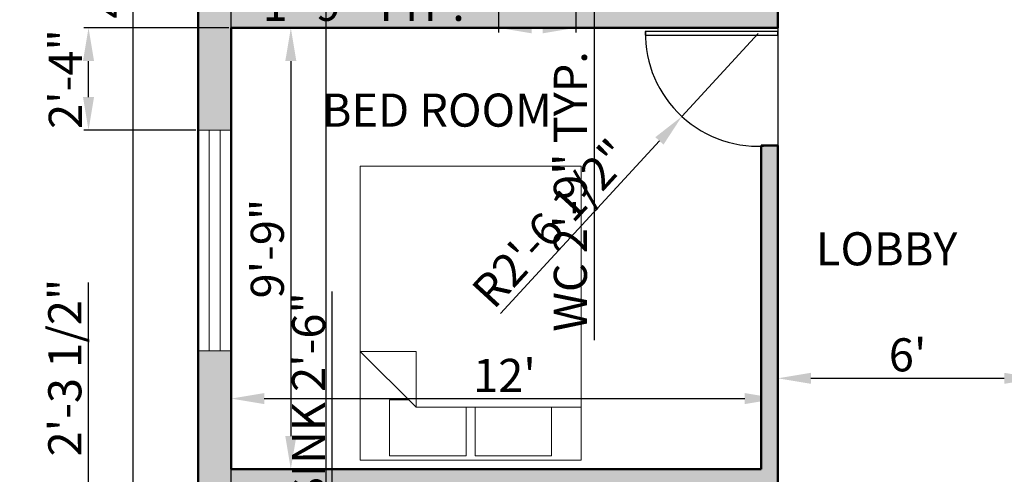
# Model space of a CAD drawing. Units: inches. Extents: x 875413 to 876020, y 447446 to 448210.
# Tile 2 of 8: x 875413 to 875681, y 447671 to 447795. Entities that reach past the tile are written whole.
import ezdxf

# ---------------------------------------------------------------- set-up
doc = ezdxf.new("R2010")
doc.units = ezdxf.units.IN
for name, color, linetype, lineweight in [('A-ANNO-DIMS', 2, 'Continuous', 13), ('A-AREA-IDEN', 7, 'Continuous', 25), ('A-DOOR', 3, 'Continuous', 25), ('A-FURN', 8, 'Continuous', 18), ('A-GLAZ', 4, 'Continuous', 20), ('A-WALL', 7, 'Continuous', 50)]:
    doc.layers.add(name, color=color, linetype=linetype, lineweight=lineweight)
doc.layers.add('A-WALL-PATT', color=18, linetype='Continuous', lineweight=13, true_color=0x000000)
doc.styles.get("Standard").update_dxf_attribs({"font": 'arial.ttf'})
doc.dimstyles.new('ISO-25', dxfattribs={"dimtxt": 9, "dimasz": 9, "dimexe": 1.25, "dimexo": 0.625, "dimtad": 1, "dimdec": 1, "dimrnd": 9, "dimlunit": 3, "dimtxsty": 'Standard', "dimcen": 2.5, "dimadec": 0, "dimazin": 0, "dimtfac": 1, "dimtdec": 1, "dimtmove": 0, "dimatfit": 3, "dimfxl": 1, "dimarcsym": 0})

# ---------------------------------------------------------------- blocks, each defined once
blk = doc.blocks.new('*D15')
at = {"layer": 'A-ANNO-DIMS', "color": 0, "lineweight": -2, "transparency": 16777216}
for p, q in [((875470.7, 447791.89), (875470.7, 447690.48)), ((875619.2, 447791.89), (875619.2, 447690.48)), ((875479.7, 447691.73), (875610.2, 447691.73))]:
    blk.add_line(p, q, dxfattribs=at)
at = {"layer": 'A-ANNO-DIMS', "color": 0, "transparency": 16777216}
for points in [[(875479.7, 447693.23), (875479.7, 447690.23), (875470.7, 447691.73)], [(875610.2, 447693.23), (875610.2, 447690.23), (875619.2, 447691.73)]]:
    blk.add_solid(points, dxfattribs=at)
at = {"layer": 'Defpoints', "color": 0, "transparency": 16777216}
for p in [(875470.7, 447792.52), (875619.2, 447792.52), (875619.2, 447691.73)]:
    blk.add_point(p, dxfattribs=at)
at = {"layer": 'A-ANNO-DIMS', "color": 0, "transparency": 16777216, "insert": (875544.95, 447696.87), "char_height": 9, "attachment_point": 5}
blk.add_mtext("12'", dxfattribs=at)
blk = doc.blocks.new('*D16')
at = {"layer": 'A-ANNO-DIMS', "color": 0, "lineweight": -2, "transparency": 16777216}
for p, q in [((875471.33, 447792.52), (875488.15, 447792.52)), ((875486.9, 447783.52), (875486.9, 447681.52)), ((875471.33, 447672.52), (875488.15, 447672.52))]:
    blk.add_line(p, q, dxfattribs=at)
at = {"layer": 'A-ANNO-DIMS', "color": 0, "transparency": 16777216}
for points in [[(875485.4, 447783.52), (875488.4, 447783.52), (875486.9, 447792.52)], [(875485.4, 447681.52), (875488.4, 447681.52), (875486.9, 447672.52)]]:
    blk.add_solid(points, dxfattribs=at)
at = {"layer": 'Defpoints', "color": 0, "transparency": 16777216}
for p in [(875470.7, 447792.52), (875470.7, 447672.52), (875486.9, 447672.52)]:
    blk.add_point(p, dxfattribs=at)
at = {"layer": 'A-ANNO-DIMS', "color": 0, "transparency": 16777216, "insert": (875481.68, 447732.52), "char_height": 9, "attachment_point": 5, "rotation": 90}
blk.add_mtext('9\'-9"', dxfattribs=at)
blk = doc.blocks.new('Bed - Queen')
for p, q in [((0, -80.00003), (0, 0)), ((0, 0), (59.99999, 0)), ((59.99999, 0), (59.99999, -80.00003)), ((7.99999, -1.2), (28.79998, -1.2)), ((7.99999, -14.4), (7.99999, -1.2)), ((28.79998, -1.2), (28.79998, -14.4)), ((31.19999, -1.2), (51.99999, -1.2)), ((31.19999, -14.4), (31.19999, -1.2)), ((51.99999, -1.2), (51.99999, -16.4)), ((0, -14.4), (44.8, -14.4)), ((59.99999, -29.6), (44.8, -14.4)), ((44.8, -14.4), (44.8, -29.6)), ((44.8, -16.8), (0, -16.8)), ((51.99999, -16.4), (46.79936, -16.4)), ((44.8, -29.6), (59.99999, -29.6)), ((59.99999, -80.00003), (0, -80.00003))]:
    blk.add_line(p, q)
blk = doc.blocks.new('*D36')
at = {"layer": 'A-ANNO-DIMS', "color": 0, "lineweight": -2, "transparency": 16777216}
for p, q in [((875619.2, 447691.1), (875619.2, 447698.49)), ((875628.2, 447697.24), (875680.7, 447697.24)), ((875689.7, 447691.1), (875689.7, 447698.49))]:
    blk.add_line(p, q, dxfattribs=at)
at = {"layer": 'A-ANNO-DIMS', "color": 0, "transparency": 16777216}
for points in [[(875628.2, 447698.74), (875628.2, 447695.74), (875619.2, 447697.24)], [(875680.7, 447698.74), (875680.7, 447695.74), (875689.7, 447697.24)]]:
    blk.add_solid(points, dxfattribs=at)
at = {"layer": 'Defpoints', "color": 0, "transparency": 16777216}
for p in [(875689.7, 447697.24), (875619.2, 447690.48), (875689.7, 447690.48)]:
    blk.add_point(p, dxfattribs=at)
at = {"layer": 'A-ANNO-DIMS', "color": 0, "transparency": 16777216, "insert": (875654.45, 447702.46), "char_height": 9, "attachment_point": 5}
blk.add_mtext("6'", dxfattribs=at)
blk = doc.blocks.new('*D38')
at = {"layer": 'A-ANNO-DIMS', "color": 0, "lineweight": -2, "transparency": 16777216}
for p, q in [((875461.08, 448079.02), (875442.76, 448079.02)), ((875444.01, 448070.02), (875444.01, 447554.02)), ((875461.08, 447545.02), (875442.76, 447545.02))]:
    blk.add_line(p, q, dxfattribs=at)
at = {"layer": 'A-ANNO-DIMS', "color": 0, "transparency": 16777216}
for points in [[(875442.51, 448070.02), (875445.51, 448070.02), (875444.01, 448079.02)], [(875442.51, 447554.02), (875445.51, 447554.02), (875444.01, 447545.02)]]:
    blk.add_solid(points, dxfattribs=at)
at = {"layer": 'Defpoints', "color": 0, "transparency": 16777216}
for p in [(875461.7, 448079.02), (875444.01, 447545.02), (875461.7, 447545.02)]:
    blk.add_point(p, dxfattribs=at)
at = {"layer": 'A-ANNO-DIMS', "color": 0, "transparency": 16777216, "insert": (875438.78, 447812.02), "char_height": 9, "attachment_point": 5, "rotation": 90}
blk.add_mtext('44\'-3"', dxfattribs=at)
blk = doc.blocks.new('WIN-60IN')
for p, q in [((0, 9), (0, 0)), ((60, 9), (60, 0)), ((60, 6), (0, 6)), ((60, 3), (0, 3))]:
    blk.add_line(p, q)
blk = doc.blocks.new('*D49')
at = {"layer": 'A-ANNO-DIMS', "color": 0, "lineweight": -2, "transparency": 16777216}
for p, q in [((875564.95, 447830.56), (875570.53, 447830.56)), ((875569.28, 447821.56), (875569.28, 447806.52)), ((875564.95, 447797.52), (875570.53, 447797.52)), ((875569.28, 447797.52), (875569.28, 447707.6))]:
    blk.add_line(p, q, dxfattribs=at)
at = {"layer": 'A-ANNO-DIMS', "color": 0, "transparency": 16777216}
for points in [[(875567.78, 447821.56), (875570.78, 447821.56), (875569.28, 447830.56)], [(875567.78, 447806.52), (875570.78, 447806.52), (875569.28, 447797.52)]]:
    blk.add_solid(points, dxfattribs=at)
at = {"layer": 'Defpoints', "color": 0, "transparency": 16777216}
for p in [(875564.32, 447830.56), (875564.32, 447797.52), (875569.28, 447797.52)]:
    blk.add_point(p, dxfattribs=at)
at = {"layer": 'A-ANNO-DIMS', "color": 0, "transparency": 16777216, "insert": (875564, 447748.06), "char_height": 9, "attachment_point": 5, "rotation": 90}
blk.add_mtext('WC 2\'-9" TYP.', dxfattribs=at)
blk = doc.blocks.new('*D50')
at = {"layer": 'A-ANNO-DIMS', "color": 0, "lineweight": -2, "transparency": 16777216}
for p, q in [((875543.32, 447796.89), (875543.32, 447791.31)), ((875564.32, 447796.89), (875564.32, 447791.31)), ((875543.32, 447792.56), (875479.06, 447792.56)), ((875555.32, 447792.56), (875552.32, 447792.56))]:
    blk.add_line(p, q, dxfattribs=at)
at = {"layer": 'A-ANNO-DIMS', "color": 0, "transparency": 16777216}
for points in [[(875552.32, 447794.06), (875552.32, 447791.06), (875543.32, 447792.56)], [(875555.32, 447794.06), (875555.32, 447791.06), (875564.32, 447792.56)]]:
    blk.add_solid(points, dxfattribs=at)
at = {"layer": 'Defpoints', "color": 0, "transparency": 16777216}
for p in [(875543.32, 447797.52), (875564.32, 447797.52), (875543.32, 447792.56)]:
    blk.add_point(p, dxfattribs=at)
at = {"layer": 'A-ANNO-DIMS', "color": 0, "transparency": 16777216, "insert": (875506.69, 447797.78), "char_height": 9, "attachment_point": 5}
blk.add_mtext('1\'-9" TYP.', dxfattribs=at)
blk = doc.blocks.new('*D65')
at = {"layer": 'A-ANNO-DIMS', "color": 0, "lineweight": -2, "transparency": 16777216}
for p, q in [((875498.17, 447653.89), (875498.17, 447720.86)), ((875494.3, 447653.89), (875499.42, 447653.89)), ((875498.17, 447632.89), (875498.17, 447644.89)), ((875494.3, 447623.89), (875499.42, 447623.89))]:
    blk.add_line(p, q, dxfattribs=at)
at = {"layer": 'A-ANNO-DIMS', "color": 0, "transparency": 16777216}
for points in [[(875496.67, 447644.89), (875499.67, 447644.89), (875498.17, 447653.89)], [(875496.67, 447632.89), (875499.67, 447632.89), (875498.17, 447623.89)]]:
    blk.add_solid(points, dxfattribs=at)
at = {"layer": 'Defpoints', "color": 0, "transparency": 16777216}
for p in [(875493.67, 447653.89), (875498.17, 447653.89), (875493.67, 447623.89)]:
    blk.add_point(p, dxfattribs=at)
at = {"layer": 'A-ANNO-DIMS', "color": 0, "transparency": 16777216, "insert": (875492.89, 447691.87), "char_height": 9, "attachment_point": 5, "rotation": 90}
blk.add_mtext('SINK 2\'-6"', dxfattribs=at)
blk = doc.blocks.new('*D72')
at = {"layer": 'A-ANNO-DIMS', "color": 0, "lineweight": -2, "transparency": 16777216}
for p, q in [((875470.08, 447792.52), (875430.7, 447792.52)), ((875431.95, 447773.71), (875431.95, 447783.52)), ((875461.08, 447764.71), (875430.7, 447764.71))]:
    blk.add_line(p, q, dxfattribs=at)
at = {"layer": 'A-ANNO-DIMS', "color": 0, "transparency": 16777216}
for points in [[(875430.45, 447783.52), (875433.45, 447783.52), (875431.95, 447792.52)], [(875430.45, 447773.71), (875433.45, 447773.71), (875431.95, 447764.71)]]:
    blk.add_solid(points, dxfattribs=at)
at = {"layer": 'Defpoints', "color": 0, "transparency": 16777216}
for p in [(875431.95, 447792.52), (875470.7, 447792.52), (875461.7, 447764.71)]:
    blk.add_point(p, dxfattribs=at)
at = {"layer": 'A-ANNO-DIMS', "color": 0, "transparency": 16777216, "insert": (875426.81, 447778.62), "char_height": 9, "attachment_point": 5, "rotation": 90}
blk.add_mtext('2\'-4"', dxfattribs=at)
blk = doc.blocks.new('*D73')
at = {"layer": 'A-ANNO-DIMS', "color": 0, "lineweight": -2, "transparency": 16777216}
for p, q in [((875431.95, 447668.02), (875431.95, 447723.32)), ((875470.08, 447668.02), (875430.7, 447668.02)), ((875431.95, 447649.7), (875431.95, 447659.02)), ((875461.08, 447640.7), (875430.7, 447640.7))]:
    blk.add_line(p, q, dxfattribs=at)
at = {"layer": 'A-ANNO-DIMS', "color": 0, "transparency": 16777216}
for points in [[(875430.45, 447659.02), (875433.45, 447659.02), (875431.95, 447668.02)], [(875430.45, 447649.7), (875433.45, 447649.7), (875431.95, 447640.7)]]:
    blk.add_solid(points, dxfattribs=at)
at = {"layer": 'Defpoints', "color": 0, "transparency": 16777216}
for p in [(875431.95, 447668.02), (875470.7, 447668.02), (875461.7, 447640.7)]:
    blk.add_point(p, dxfattribs=at)
at = {"layer": 'A-ANNO-DIMS', "color": 0, "transparency": 16777216, "insert": (875426.67, 447700.17), "char_height": 9, "attachment_point": 5, "rotation": 90}
blk.add_mtext('2\'-3 1/2"', dxfattribs=at)
blk = doc.blocks.new('*D82')
at = {"layer": 'A-ANNO-DIMS', "color": 0, "lineweight": -2, "transparency": 16777216}
for p, q in [((875470.7, 447554.64), (875470.7, 448110.02)), ((875487.52, 448108.77), (875479.7, 448108.77)), ((875496.52, 447585.21), (875496.52, 448110.02))]:
    blk.add_line(p, q, dxfattribs=at)
at = {"layer": 'A-ANNO-DIMS', "color": 0, "transparency": 16777216}
for points in [[(875479.7, 448110.27), (875479.7, 448107.27), (875470.7, 448108.77)], [(875487.52, 448110.27), (875487.52, 448107.27), (875496.52, 448108.77)]]:
    blk.add_solid(points, dxfattribs=at)
at = {"layer": 'Defpoints', "color": 0, "transparency": 16777216}
for p in [(875470.7, 448108.77), (875496.52, 447584.59), (875470.7, 447554.02)]:
    blk.add_point(p, dxfattribs=at)
at = {"layer": 'A-ANNO-DIMS', "color": 0, "transparency": 16777216, "insert": (875483.61, 448113.91), "char_height": 9, "attachment_point": 5}
blk.add_mtext('2\'-2"', dxfattribs=at)
blk = doc.blocks.new('*D98')
at = {"layer": 'A-ANNO-DIMS', "color": 0, "lineweight": -2, "transparency": 16777216}
for p, q in [((875613.86, 447791.02), (875593.12, 447768.44)), ((875543.89, 447714.86), (875587.03, 447761.81))]:
    blk.add_line(p, q, dxfattribs=at)
at = {"layer": 'A-ANNO-DIMS', "color": 0, "transparency": 16777216}
blk.add_solid([(875585.92, 447762.82), (875588.13, 447760.79), (875593.12, 447768.44)], dxfattribs=at)
at = {"layer": 'Defpoints', "color": 0, "transparency": 16777216}
for p in [(875613.86, 447791.02), (875593.12, 447768.44)]:
    blk.add_point(p, dxfattribs=at)
at = {"layer": 'A-ANNO-DIMS', "color": 0, "transparency": 16777216, "insert": (875558.53, 447738.59), "char_height": 9, "attachment_point": 5, "rotation": 47.4249}
blk.add_mtext('R2\'-6 1/2"', dxfattribs=at)

msp = doc.modelspace()

# ---------------------------------------------------------------- hatches: boundary and pattern name
at = {"layer": 'A-WALL-PATT'}
h = msp.add_hatch(color=256, dxfattribs=at)
h.dxf.hatch_style = 1
h.paths.add_polyline_path([(875470.7, 447985.13), (875461.7, 447985.13), (875461.7, 447865.29), (875470.7, 447865.29), (875470.7, 447881.02), (875566.7, 447881.02), (875566.7, 447797.02), (875571.2, 447797.02), (875571.2, 447885.52), (875571.2, 447921.52), (875603.29, 447921.52), (875603.29, 447926.02), (875501.27, 447926.02), (875501.27, 447921.52), (875566.7, 447921.52), (875566.7, 447885.52), (875470.7, 447885.52), (875470.7, 447921.52), (875470.7, 447926.02)])
h.paths.add_polyline_path([(875470.7, 448070.02), (875518.96, 448070.02), (875518.96, 448079.02), (875461.7, 448079.02), (875461.7, 448045.13), (875470.7, 448045.13)])
h.paths.add_polyline_path([(875819.9, 448079.02), (875578.96, 448079.02), (875578.96, 448070.02), (875638.7, 448070.02), (875638.7, 447921.52), (875643.2, 447921.52), (875643.2, 448070.02), (875763.2, 448070.02), (875763.2, 447921.52), (875767.7, 447921.52), (875767.7, 448070.02), (875819.9, 448070.02)])
h.paths.add_polyline_path([(875935.7, 447978.92), (875926.7, 447978.92), (875926.7, 447926.02), (875926.7, 447921.52), (875926.7, 447885.52), (875842.7, 447885.52), (875842.7, 447921.52), (875899.7, 447921.52), (875899.7, 447926.02), (875805.34, 447926.02), (875805.34, 447921.52), (875838.2, 447921.52), (875838.2, 447885.52), (875838.2, 447797.02), (875689.7, 447797.02), (875689.7, 447792.52), (875842.7, 447792.52), (875842.7, 447881.02), (875926.7, 447881.02), (875926.7, 447857.16), (875935.7, 447857.16)])
h.paths.add_polyline_path([(875935.7, 448079.02), (875879.9, 448079.02), (875879.9, 448070.02), (875926.7, 448070.02), (875926.7, 448038.92), (875935.7, 448038.92)])
h.paths.add_polyline_path([(875935.7, 447833.16), (875926.7, 447833.16), (875926.7, 447797.02), (875842.7, 447797.02), (875842.7, 447792.52), (875926.7, 447792.52), (875926.7, 447756.52), (875935.7, 447756.52)])
h.paths.add_polyline_path([(875935.7, 447732.52), (875926.7, 447732.52), (875926.7, 447692.75, -0.007222), (875926.81, 447692.41, -0.08192), (875927.45, 447687.6, -0.071798), (875926.7, 447683.4), (875926.7, 447672.52), (875808.63, 447672.52), (875808.63, 447668.02), (875926.7, 447668.02), (875926.7, 447663.19), (875935.7, 447663.19)])
h.paths.add_polyline_path([(875842.7, 447792.52), (875838.2, 447792.52), (875838.2, 447704.02), (875842.7, 447704.02)])
h.paths.add_polyline_path([(875470.7, 447792.52), (875619.2, 447792.52), (875619.2, 447797.02), (875470.7, 447797.02), (875470.7, 447841.29), (875461.7, 447841.29), (875461.7, 447764.71), (875470.7, 447764.71)])
h.paths.add_polyline_path([(875619.2, 447760.51), (875616.95, 447760.51, -0.018388), (875614.7, 447760.37), (875614.7, 447672.52), (875470.7, 447672.52), (875470.7, 447704.71), (875461.7, 447704.71), (875461.7, 447640.7), (875470.7, 447640.7), (875470.7, 447668.02), (875619.2, 447668.02)])
h.paths.add_polyline_path([(875511.12, 447554.02), (875470.7, 447554.02), (875470.7, 447580.7), (875461.7, 447580.7), (875461.7, 447545.02), (875511.12, 447545.02)])
h.paths.add_polyline_path([(875656.47, 447554.02), (875620.05, 447554.02, -0.057036), (875616.67, 447553.74, -0.040891), (875614.26, 447554.02), (875571.12, 447554.02), (875571.12, 447545.02), (875656.47, 447545.02)])
h.paths.add_polyline_path([(875643.2, 447613.27), (875685.21, 447613.27), (875685.21, 447617.77), (875685.21, 447623.8), (875680.71, 447623.8), (875680.71, 447617.77), (875618.23, 447617.77), (875618.23, 447623.8), (875613.73, 447623.8), (875613.73, 447617.77), (875613.73, 447613.27), (875638.7, 447613.27), (875638.7, 447554.02), (875643.2, 447554.02)])
h.paths.add_polyline_path([(875694.2, 447760.28), (875689.7, 447760.28), (875689.7, 447668.02), (875748.63, 447668.02), (875748.63, 447672.52), (875694.2, 447672.52)])

# ---------------------------------------------------------------- linework, layer by layer
at = {"layer": 'A-DOOR'}
for p, q in [((875619.2, 447792.52), (875619.2, 447791.52)), ((875619.2, 447791.52), (875583.2, 447791.52)), ((875583.2, 447791.52), (875583.2, 447790.52)), ((875583.2, 447790.52), (875619.2, 447790.52)), ((875619.2, 447790.52), (875619.2, 447791.52))]:
    msp.add_line(p, q, dxfattribs=at)
msp.add_arc((875613.86, 447791.02), 30.66, 179.0657, 275.7843, dxfattribs=at)
at = {"layer": 'A-WALL'}
for p, q in [((875461.7, 448079.02), (875461.7, 447545.02)), ((875619.2, 447797.02), (875619.2, 447792.52)), ((875470.7, 447792.52), (875470.7, 447672.52)), ((875619.2, 447792.52), (875470.7, 447792.52)), ((875614.7, 447760.51), (875614.7, 447672.52)), ((875619.2, 447760.51), (875614.7, 447760.51)), ((875619.2, 447760.51), (875619.2, 447668.02)), ((875614.7, 447672.52), (875470.7, 447672.52))]:
    msp.add_line(p, q, dxfattribs=at)

# ---------------------------------------------------------------- block references
at = {"layer": 'A-FURN', "rotation": 180}
msp.add_blockref('Bed - Queen', (875565.75, 447674.96), dxfattribs=at)
at = {"layer": 'A-GLAZ', "rotation": 269.9999999998478}
msp.add_blockref('WIN-60IN', (875461.7, 447764.71), dxfattribs=at)

# ---------------------------------------------------------------- texts
at = {"layer": 'A-AREA-IDEN', "char_height": 9, "attachment_point": 1}
for s, insert in [('BED ROOM', (875495.31, 447774.67)), ('LOBBY', (875629.54, 447736.96))]:
    msp.add_mtext_dynamic_manual_height_columns(s, width=100.7812, gutter_width=12.5, heights=[0], dxfattribs=dict(at, insert=insert))

# ---------------------------------------------------------------- dimensions: what is measured, and where the dimension line sits
at = {"layer": 'A-ANNO-DIMS'}
for base, p1, p2, override, picture, middle in [((875470.7, 448108.77), (875496.52, 447584.59), (875470.7, 447554.02), {"dimdec": 1, "dimlfac": 1, "dimrnd": 0, "dimzin": 1, "dimdsep": 46, "dimlunit": 4, "dimfrac": 2}, '*D82', (875483.61, 448113.91)), ((875619.2, 447691.73), (875470.7, 447792.52), (875619.2, 447792.52), {"dimclrd": 0, "dimclre": 0, "dimclrt": 0}, '*D15', (875544.95, 447696.87)), ((875689.7, 447697.24), (875619.2, 447690.48), (875689.7, 447690.48), {"dimclrd": 0, "dimclre": 0, "dimclrt": 0}, '*D36', (875654.45, 447702.46))]:
    dim = msp.add_linear_dim(base=base, p1=p1, p2=p2, dimstyle='ISO-25', override=override, dxfattribs=at)
    dim.commit()
    dim.dimension.update_dxf_attribs({"geometry": picture, "text_midpoint": middle})
for base, p1, p2, override, picture, middle in [((875444.01, 447545.02), (875461.7, 448079.02), (875461.7, 447545.02), {"dimclrd": 0, "dimclre": 0, "dimclrt": 0}, '*D38', (875438.78, 447812.02)), ((875431.95, 447792.52), (875461.7, 447764.71), (875470.7, 447792.52), {"dimdec": 1, "dimlfac": 1, "dimrnd": 0, "dimzin": 1, "dimdsep": 46, "dimlunit": 4, "dimfrac": 2}, '*D72', (875426.81, 447778.62)), ((875486.9, 447672.52), (875470.7, 447792.52), (875470.7, 447672.52), {"dimclrd": 0, "dimclre": 0, "dimclrt": 0}, '*D16', (875481.68, 447732.52)), ((875431.95, 447668.02), (875461.7, 447640.7), (875470.7, 447668.02), {"dimdec": 1, "dimlfac": 1, "dimrnd": 0, "dimzin": 1, "dimdsep": 46, "dimlunit": 4, "dimfrac": 2}, '*D73', (875426.67, 447700.17))]:
    dim = msp.add_linear_dim(base=base, p1=p1, p2=p2, angle=90, dimstyle='ISO-25', override=override, dxfattribs=at)
    dim.commit()
    dim.dimension.update_dxf_attribs({"geometry": picture, "text_midpoint": middle})
for base, p1, p2, angle, text, picture, middle in [((875569.28, 447797.52), (875564.32, 447830.56), (875564.32, 447797.52), 270, 'WC <> TYP.', '*D49', (875564, 447748.06)), ((875543.32, 447792.56), (875564.32, 447797.52), (875543.32, 447797.52), 180, '<> TYP.', '*D50', (875506.69, 447797.78)), ((875498.17, 447653.89), (875493.67, 447623.89), (875493.67, 447653.89), 90, 'SINK <>', '*D65', (875492.89, 447691.87))]:
    dim = msp.add_linear_dim(base=base, p1=p1, p2=p2, angle=angle, text=text, dimstyle='ISO-25', override={"dimdec": 1, "dimlfac": 1, "dimrnd": 0, "dimzin": 1, "dimdsep": 46, "dimlunit": 4, "dimfrac": 2}, dxfattribs=at)
    dim.commit()
    dim.dimension.update_dxf_attribs({"geometry": picture, "text_midpoint": middle})
dim = msp.add_radius_dim(center=(875613.86, 447791.02), mpoint=(875593.12, 447768.44), dimstyle='ISO-25', override={"dimdec": 1, "dimlfac": 1, "dimrnd": 0, "dimzin": 1, "dimdsep": 46, "dimlunit": 4, "dimfrac": 2}, dxfattribs=at)
dim.commit()
dim.dimension.update_dxf_attribs({"geometry": '*D98', "text_midpoint": (875558.53, 447738.59)})

doc.saveas('drawing.dxf')
